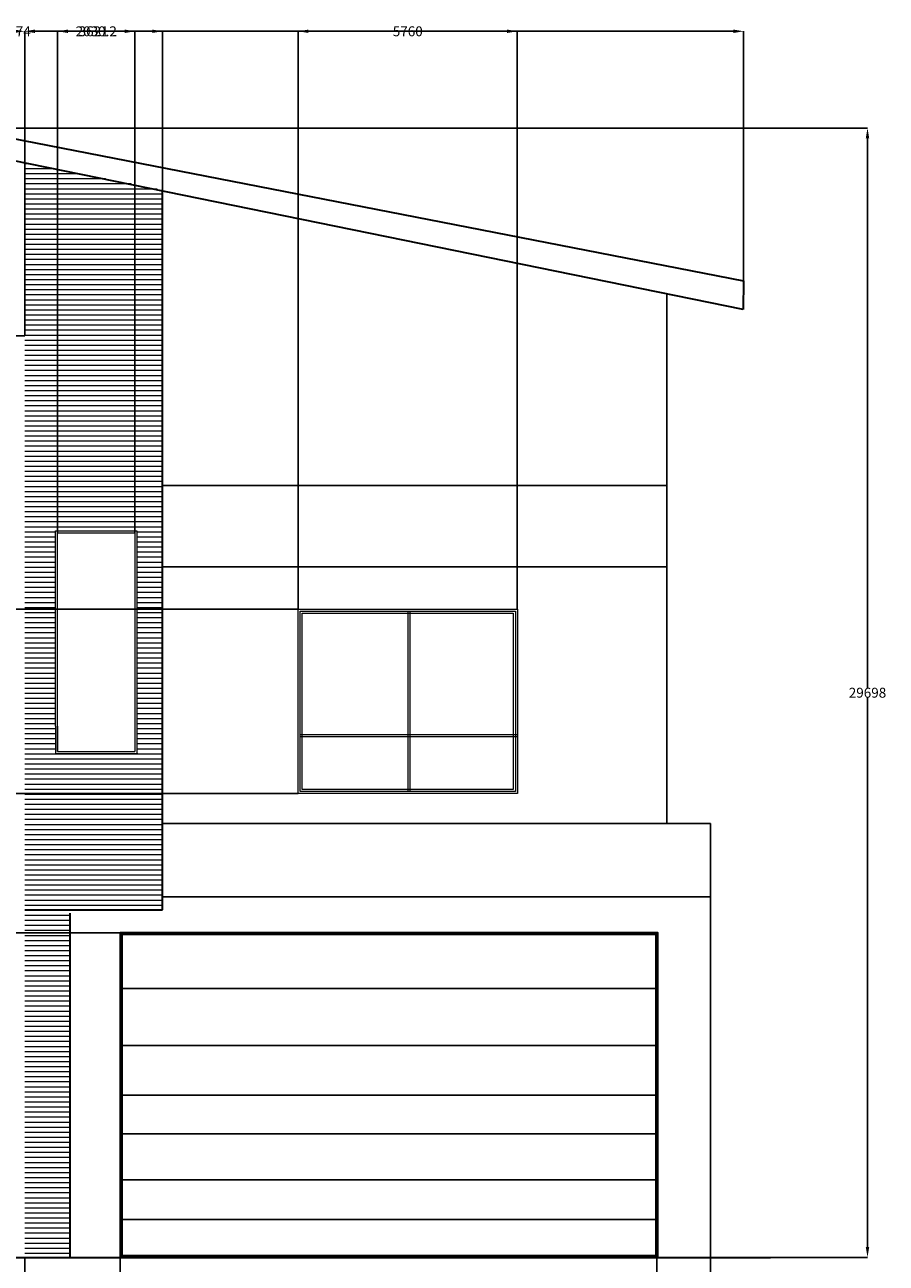
# Model space of a CAD drawing. Units: millimetres. Extents: x 23 to 3809233, y 4 to 290343.
# Tile 8 of 8: x 1921861 to 1944512, y 173128 to 205695. Entities that reach past the tile are written whole.
import ezdxf

# ---------------------------------------------------------------- set-up
doc = ezdxf.new("R2010")
doc.units = ezdxf.units.MM
doc.header["$MEASUREMENT"] = 0
for name, color, linetype, lineweight in [('A-ANNO-DIMS', 2, 'Continuous', 18), ('A-COLS', 7, 'Continuous', 35), ('A-DOOR', 3, 'Continuous', 25), ('A-ELEV', 7, 'Continuous', 25), ('A-ELEV-GRND', 7, 'Continuous', 30), ('A-GLAZ', 4, 'Continuous', 18), ('A-ROOF', 7, 'Continuous', 35), ('A-WALL-PATT', 252, 'Continuous', 13)]:
    doc.layers.add(name, color=color, linetype=linetype, lineweight=lineweight)
doc.styles.get("Standard").update_dxf_attribs({"font": 'arial.ttf'})
doc.dimstyles.get("Standard").update_dxf_attribs({"dimtxt": 260.18, "dimasz": 270.18, "dimexe": 0.18, "dimexo": 0.0625, "dimgap": 0.09, "dimtad": 0, "dimtih": 1, "dimtoh": 1, "dimdec": 0, "dimzin": 0, "dimdsep": 46, "dimtxsty": 'Standard', "dimcen": 0.09, "dimadec": 0, "dimazin": 0, "dimtfac": 1, "dimtdec": 0, "dimtofl": 0, "dimtmove": 0, "dimatfit": 3, "dimfxl": 1, "dimtolj": 1, "dimtzin": 0, "dimarcsym": 0})

# ---------------------------------------------------------------- blocks, each defined once
blk = doc.blocks.new('*D94')
at = {"layer": 'A-ANNO-DIMS', "color": 0, "lineweight": -2, "transparency": 16777216}
for p, q in [((1902289, 186535), (1902289, 205525)), ((1902560, 205524), (1921037, 205524)), ((1940493, 205524), (1922015, 205524)), ((1940763, 198959), (1940763, 205525))]:
    blk.add_line(p, q, dxfattribs=at)
at = {"layer": 'A-ANNO-DIMS', "color": 0, "transparency": 16777216}
for points in [[(1902560, 205569), (1902560, 205479), (1902289, 205524)], [(1940493, 205569), (1940493, 205479), (1940763, 205524)]]:
    blk.add_solid(points, dxfattribs=at)
at = {"layer": 'Defpoints', "color": 0, "transparency": 16777216}
for p in [(1940763, 205524), (1940763, 198959), (1902289, 186535)]:
    blk.add_point(p, dxfattribs=at)
at = {"layer": 'A-ANNO-DIMS', "color": 0, "transparency": 16777216, "insert": (1921526, 205524), "char_height": 260.2, "attachment_point": 5}
blk.add_mtext('\\A1;38474', dxfattribs=at)
blk = doc.blocks.new('*D95')
at = {"layer": 'A-ANNO-DIMS', "color": 0, "lineweight": -2, "transparency": 16777216}
for p, q in [((1920137, 202978), (1944019, 202978)), ((1944019, 202708), (1944019, 188263)), ((1944019, 173551), (1944019, 187997)), ((1939891, 173281), (1944019, 173281))]:
    blk.add_line(p, q, dxfattribs=at)
at = {"layer": 'A-ANNO-DIMS', "color": 0, "transparency": 16777216}
for points in [[(1943974, 202708), (1944064, 202708), (1944019, 202978)], [(1943974, 173551), (1944064, 173551), (1944019, 173281)]]:
    blk.add_solid(points, dxfattribs=at)
at = {"layer": 'Defpoints', "color": 0, "transparency": 16777216}
for p in [(1920137, 202978), (1944019, 202978), (1939891, 173281)]:
    blk.add_point(p, dxfattribs=at)
at = {"layer": 'A-ANNO-DIMS', "color": 0, "transparency": 16777216, "insert": (1944019, 188130), "char_height": 260.2, "attachment_point": 5}
blk.add_mtext('\\A1;29698', dxfattribs=at)
blk = doc.blocks.new('*D99')
at = {"layer": 'A-ANNO-DIMS', "color": 0, "lineweight": -2, "transparency": 16777216}
for p, q in [((1921861, 173281), (1921861, 166038)), ((1924370, 173282), (1924370, 166038)), ((1922131, 166038), (1922572, 166038)), ((1924100, 166038), (1923659, 166038))]:
    blk.add_line(p, q, dxfattribs=at)
at = {"layer": 'A-ANNO-DIMS', "color": 0, "transparency": 16777216}
for points in [[(1922131, 166083), (1922131, 165993), (1921861, 166038)], [(1924100, 166083), (1924100, 165993), (1924370, 166038)]]:
    blk.add_solid(points, dxfattribs=at)
at = {"layer": 'Defpoints', "color": 0, "transparency": 16777216}
for p in [(1921861, 173281), (1924370, 173282), (1924370, 166038)]:
    blk.add_point(p, dxfattribs=at)
at = {"layer": 'A-ANNO-DIMS', "color": 0, "transparency": 16777216, "insert": (1923116, 166038), "char_height": 260.2, "attachment_point": 5}
blk.add_mtext('\\A1;2509.5', dxfattribs=at)
blk = doc.blocks.new('*D100')
at = {"layer": 'A-ANNO-DIMS', "color": 0, "lineweight": -2, "transparency": 16777216}
for p, q in [((1924370, 173282), (1924370, 166038)), ((1938484, 173307), (1938484, 166038)), ((1924641, 166038), (1930950, 166038)), ((1938214, 166038), (1931904, 166038))]:
    blk.add_line(p, q, dxfattribs=at)
at = {"layer": 'A-ANNO-DIMS', "color": 0, "transparency": 16777216}
for points in [[(1924641, 166083), (1924641, 165993), (1924370, 166038)], [(1938214, 166083), (1938214, 165993), (1938484, 166038)]]:
    blk.add_solid(points, dxfattribs=at)
at = {"layer": 'Defpoints', "color": 0, "transparency": 16777216}
for p in [(1924370, 173282), (1938484, 173307), (1938484, 166038)]:
    blk.add_point(p, dxfattribs=at)
at = {"layer": 'A-ANNO-DIMS', "color": 0, "transparency": 16777216, "insert": (1931427, 166038), "char_height": 260.2, "attachment_point": 5}
blk.add_mtext('\\A1;14114', dxfattribs=at)
blk = doc.blocks.new('*D101')
at = {"layer": 'A-ANNO-DIMS', "color": 0, "lineweight": -2, "transparency": 16777216}
for p, q in [((1938484, 173307), (1938484, 166038)), ((1939891, 173281), (1939891, 166038)), ((1938214, 166038), (1937944, 166038)), ((1940162, 166038), (1940432, 166038))]:
    blk.add_line(p, q, dxfattribs=at)
at = {"layer": 'A-ANNO-DIMS', "color": 0, "transparency": 16777216}
for points in [[(1938214, 166083), (1938214, 165993), (1938484, 166038)], [(1940162, 166083), (1940162, 165993), (1939891, 166038)]]:
    blk.add_solid(points, dxfattribs=at)
at = {"layer": 'Defpoints', "color": 0, "transparency": 16777216}
for p in [(1938484, 173307), (1939891, 173281), (1939891, 166038)]:
    blk.add_point(p, dxfattribs=at)
at = {"layer": 'A-ANNO-DIMS', "color": 0, "transparency": 16777216, "insert": (1939188, 166038), "char_height": 260.2, "attachment_point": 5}
blk.add_mtext('\\A1;1407.4', dxfattribs=at)
blk = doc.blocks.new('*D104')
at = {"layer": 'A-ANNO-DIMS', "color": 0, "lineweight": -2, "transparency": 16777216}
for p, q in [((1924370.307623, 181820.425276), (1888189.886131, 181820.425276)), ((1888190.066131, 181550.245276), (1888190.066131, 177684.406757)), ((1888190.066131, 173552.529002), (1888190.066131, 177418.367521)), ((1924370.346212, 173282.349002), (1888189.886131, 173282.349002))]:
    blk.add_line(p, q, dxfattribs=at)
at = {"layer": 'A-ANNO-DIMS', "color": 0, "transparency": 16777216}
for points in [[(1888145.036131, 181550.245276), (1888235.096131, 181550.245276), (1888190.066131, 181820.425276)], [(1888145.036131, 173552.529002), (1888235.096131, 173552.529002), (1888190.066131, 173282.349002)]]:
    blk.add_solid(points, dxfattribs=at)
at = {"layer": 'Defpoints', "color": 0, "transparency": 16777216}
for p in [(1888190.066131, 181820.425276), (1924370.370123, 181820.425276), (1924370.408712, 173282.349002)]:
    blk.add_point(p, dxfattribs=at)
at = {"layer": 'A-ANNO-DIMS', "color": 0, "transparency": 16777216, "insert": (1888190.066131, 177551.387139), "char_height": 260.18, "attachment_point": 5}
blk.add_mtext('\\A1;8538', dxfattribs=at)
blk = doc.blocks.new('*D105')
at = {"layer": 'A-ANNO-DIMS', "color": 0, "lineweight": -2, "transparency": 16777216}
for p, q in [((1903366, 194022), (1903366, 205525)), ((1903636, 205524), (1912135, 205524)), ((1921591, 205524), (1913092, 205524)), ((1921861, 197518), (1921861, 205525))]:
    blk.add_line(p, q, dxfattribs=at)
at = {"layer": 'A-ANNO-DIMS', "color": 0, "transparency": 16777216}
for points in [[(1903636, 205569), (1903636, 205479), (1903366, 205524)], [(1921591, 205569), (1921591, 205479), (1921861, 205524)]]:
    blk.add_solid(points, dxfattribs=at)
at = {"layer": 'Defpoints', "color": 0, "transparency": 16777216}
for p in [(1921861, 205524), (1921861, 197518), (1903366, 194022)]:
    blk.add_point(p, dxfattribs=at)
at = {"layer": 'A-ANNO-DIMS', "color": 0, "transparency": 16777216, "insert": (1912613, 205524), "char_height": 260.2, "attachment_point": 5}
blk.add_mtext('\\A1;18495', dxfattribs=at)
blk = doc.blocks.new('*D106')
at = {"layer": 'A-ANNO-DIMS', "color": 0, "lineweight": -2, "transparency": 16777216}
for p, q in [((1921861, 197518), (1921861, 205525)), ((1922131, 205524), (1923308, 205524)), ((1925212, 205524), (1924035, 205524)), ((1925482, 201357), (1925482, 205525))]:
    blk.add_line(p, q, dxfattribs=at)
at = {"layer": 'A-ANNO-DIMS', "color": 0, "transparency": 16777216}
for points in [[(1922131, 205569), (1922131, 205479), (1921861, 205524)], [(1925212, 205569), (1925212, 205479), (1925482, 205524)]]:
    blk.add_solid(points, dxfattribs=at)
at = {"layer": 'Defpoints', "color": 0, "transparency": 16777216}
for p in [(1925482, 205524), (1925482, 201357), (1921861, 197518)]:
    blk.add_point(p, dxfattribs=at)
at = {"layer": 'A-ANNO-DIMS', "color": 0, "transparency": 16777216, "insert": (1923671, 205524), "char_height": 260.2, "attachment_point": 5}
blk.add_mtext('\\A1;3621', dxfattribs=at)
blk = doc.blocks.new('*D107')
at = {"layer": 'A-ANNO-DIMS', "color": 0, "lineweight": -2, "transparency": 16777216}
for p, q in [((1921861, 197518), (1888190, 197518)), ((1888190, 197248), (1888190, 195903)), ((1888190, 194292), (1888190, 195637)), ((1903366, 194022), (1888190, 194022))]:
    blk.add_line(p, q, dxfattribs=at)
at = {"layer": 'A-ANNO-DIMS', "color": 0, "transparency": 16777216}
for points in [[(1888145, 197248), (1888235, 197248), (1888190, 197518)], [(1888145, 194292), (1888235, 194292), (1888190, 194022)]]:
    blk.add_solid(points, dxfattribs=at)
at = {"layer": 'Defpoints', "color": 0, "transparency": 16777216}
for p in [(1888190, 197518), (1921861, 197518), (1903366, 194022)]:
    blk.add_point(p, dxfattribs=at)
at = {"layer": 'A-ANNO-DIMS', "color": 0, "transparency": 16777216, "insert": (1888190, 195770), "char_height": 260.2, "attachment_point": 5}
blk.add_mtext('\\A1;3496.4', dxfattribs=at)
blk = doc.blocks.new('*D113')
at = {"layer": 'A-ANNO-DIMS', "color": 0, "lineweight": -2, "transparency": 16777216}
for p, q in [((1922725, 192331), (1922725, 205525)), ((1922996, 205524), (1923199, 205524)), ((1924485, 205524), (1924282, 205524)), ((1924756, 192331), (1924756, 205525))]:
    blk.add_line(p, q, dxfattribs=at)
at = {"layer": 'A-ANNO-DIMS', "color": 0, "transparency": 16777216}
for points in [[(1922996, 205569), (1922996, 205479), (1922725, 205524)], [(1924485, 205569), (1924485, 205479), (1924756, 205524)]]:
    blk.add_solid(points, dxfattribs=at)
at = {"layer": 'Defpoints', "color": 0, "transparency": 16777216}
for p in [(1924756, 205524), (1922725, 192331), (1924756, 192331)]:
    blk.add_point(p, dxfattribs=at)
at = {"layer": 'A-ANNO-DIMS', "color": 0, "transparency": 16777216, "insert": (1923740, 205524), "char_height": 260.2, "attachment_point": 5}
blk.add_mtext('\\A1;2030.2', dxfattribs=at)
blk = doc.blocks.new('*D114')
at = {"layer": 'A-ANNO-DIMS', "color": 0, "lineweight": -2, "transparency": 16777216}
for p, q in [((1929050, 190325), (1929050, 205525)), ((1929321, 205524), (1931542, 205524)), ((1934541, 205524), (1932319, 205524)), ((1934811, 190327), (1934811, 205525))]:
    blk.add_line(p, q, dxfattribs=at)
at = {"layer": 'A-ANNO-DIMS', "color": 0, "transparency": 16777216}
for points in [[(1929321, 205569), (1929321, 205479), (1929050, 205524)], [(1934541, 205569), (1934541, 205479), (1934811, 205524)]]:
    blk.add_solid(points, dxfattribs=at)
at = {"layer": 'Defpoints', "color": 0, "transparency": 16777216}
for p in [(1934811, 205524), (1929050, 190325), (1934811, 190327)]:
    blk.add_point(p, dxfattribs=at)
at = {"layer": 'A-ANNO-DIMS', "color": 0, "transparency": 16777216, "insert": (1931931, 205524), "char_height": 260.2, "attachment_point": 5}
blk.add_mtext('\\A1;5760', dxfattribs=at)
blk = doc.blocks.new('*D115')
at = {"layer": 'A-ANNO-DIMS', "color": 0, "lineweight": -2, "transparency": 16777216}
for p, q in [((1929050.318541, 190325.231012), (1888189.886131, 190325.231012)), ((1888190.066131, 190055.051012), (1888190.066131, 188036.972999)), ((1888190.066131, 185752.85575), (1888190.066131, 187770.933763)), ((1929050.318541, 185482.67575), (1888189.886131, 185482.67575))]:
    blk.add_line(p, q, dxfattribs=at)
at = {"layer": 'A-ANNO-DIMS', "color": 0, "transparency": 16777216}
for points in [[(1888145.036131, 190055.051012), (1888235.096131, 190055.051012), (1888190.066131, 190325.231012)], [(1888145.036131, 185752.85575), (1888235.096131, 185752.85575), (1888190.066131, 185482.67575)]]:
    blk.add_solid(points, dxfattribs=at)
at = {"layer": 'Defpoints', "color": 0, "transparency": 16777216}
for p in [(1888190.066131, 190325.231012), (1929050.381041, 190325.231012), (1929050.381041, 185482.67575)]:
    blk.add_point(p, dxfattribs=at)
at = {"layer": 'A-ANNO-DIMS', "color": 0, "transparency": 16777216, "insert": (1888190.066131, 187903.953381), "char_height": 260.18, "attachment_point": 5}
blk.add_mtext('\\A1;4843', dxfattribs=at)

msp = doc.modelspace()

# ---------------------------------------------------------------- hatches: boundary and pattern name
at = {"layer": 'A-WALL-PATT'}
h = msp.add_hatch(dxfattribs=at)
h.set_pattern_fill('ANSI31', color=256, scale=1061.3134, angle=-45, style=0)
h.paths.add_polyline_path([(1921860.931, 182422.235), (1925481.709, 182422.235), (1925481.709, 201356.818), (1921860.931, 202063.759)])
h.paths.add_polyline_path([(1922672.309, 192384.187), (1924806.696, 192384.187), (1924806.696, 186534.824), (1922672.309, 186534.824)], flags=0)
h = msp.add_hatch(dxfattribs=at)
h.set_pattern_fill('ANSI31', color=256, scale=1061.3134, angle=-45, style=0)
h.paths.add_polyline_path([(1921860.931, 173280.749), (1923056.615, 173280.749), (1923056.615, 182422.235), (1921860.931, 182422.235)])

# ---------------------------------------------------------------- linework, layer by layer
at = {"layer": 'A-COLS'}
for p, q in [((1925481.709, 195073.74), (1925481.709, 201356.818)), ((1925481.709, 182422.235), (1925481.709, 195073.74)), ((1921860.931, 182422.235), (1925481.709, 182422.235)), ((1923056.615, 173280.749), (1923056.615, 182330.475))]:
    msp.add_line(p, q, dxfattribs=at)
at = {"layer": 'A-DOOR'}
for p, q in [((1924423.436, 180352.795), (1938510.519, 180352.795)), ((1924370.37, 178855.255), (1938510.519, 178855.255)), ((1924423.436, 177551.582), (1938510.519, 177551.582)), ((1924396.903, 176534.585), (1938457.453, 176534.585)), ((1924396.903, 175317.891), (1938510.519, 175317.891)), ((1924423.436, 174280.085), (1938510.519, 174280.085))]:
    msp.add_line(p, q, dxfattribs=at)
msp.add_lwpolyline([(1938510.519, 173282.739, -0.414213562), (1938508.529, 173280.749), (1924372.36, 173280.749, -0.414213562), (1924370.37, 173282.739), (1924370.37, 181820.425, -0.414213562), (1924372.36, 181822.415), (1938508.529, 181822.415, -0.414213562), (1938510.519, 181820.425)], format="xyb", close=True, dxfattribs=at)
for points in [[(1938483.986, 173307.282), (1924396.903, 173307.282), (1924396.903, 181795.882), (1938483.986, 181795.882)], [(1938457.453, 173333.815), (1924423.436, 173333.815), (1924423.436, 181769.35), (1938457.453, 181769.35)]]:
    msp.add_lwpolyline(points, close=True, dxfattribs=at)
at = {"layer": 'A-ELEV'}
for p, q in [((1938740.781, 193575.546), (1938740.781, 198617.113)), ((1938740.781, 193575.546), (1925481.709, 193575.546)), ((1938740.781, 184691.073), (1938740.781, 193575.546)), ((1928568.226, 184677.526), (1928570.216, 184677.526)), ((1939891.392, 182760.245), (1925481.709, 182760.245)), ((1939891.392, 173280.749), (1939891.392, 182760.245))]:
    msp.add_line(p, q, dxfattribs=at)
msp.add_lwpolyline([(1925481.709, 191443.399), (1925481.709, 191443.399), (1938740.781, 191443.399), (1938740.781, 191443.399), (1938740.781, 191443.399), (1938740.781, 191443.399), (1925481.709, 191443.399), (1925481.709, 191443.399)], close=True, dxfattribs=at)
for points in [[(1925481.709, 184691.073), (1939889.402, 184691.073, -0.414213562), (1939891.392, 184689.083), (1939891.392, 182762.235, -0.414213562), (1939889.402, 182760.245)], [(1928572.205, 184691.073, -0.414213562), (1928570.216, 184693.063)]]:
    msp.add_lwpolyline(points, format="xyb", dxfattribs=at)
at = {"layer": 'A-ELEV-GRND'}
msp.add_line((1914495.5, 173280.749), (1941473.027, 173280.749), dxfattribs=at)
at = {"layer": 'A-GLAZ'}
for p, q in [((1924753.63, 192331.121), (1924753.63, 186587.89)), ((1931931.582, 190274.155), (1931931.582, 185533.751)), ((1931984.647, 190274.155), (1931984.647, 185533.751)), ((1922672.309, 187248.079), (1922672.309, 186534.824)), ((1922725.374, 187248.079), (1922725.374, 186587.89)), ((1924806.696, 187246.089), (1924806.696, 186534.824)), ((1929103.447, 187035.053), (1934812.782, 187035.053)), ((1929103.447, 186981.987), (1934812.782, 186981.987)), ((1922672.309, 186534.824), (1924832.632, 186534.824)), ((1922725.374, 186587.89), (1924753.63, 186587.89))]:
    msp.add_line(p, q, dxfattribs=at)
msp.add_lwpolyline([(1922674.298, 187246.089, -0.414213562), (1922672.309, 187248.079), (1922672.309, 192382.197, -0.414213562), (1922674.298, 192384.187), (1924806.696, 192384.187, -0.414213562), (1924808.686, 192382.197), (1924808.686, 187248.079, -0.414213562), (1924806.696, 187246.089)], format="xyb", dxfattribs=at)
msp.add_lwpolyline([(1922725.374, 186587.89), (1922725.374, 192331.121), (1924755.62, 192331.121), (1924755.62, 187299.154)], dxfattribs=at)
msp.add_lwpolyline([(1929050.381, 190325.231, -0.414213562), (1929052.371, 190327.221), (1934810.792, 190327.221, -0.414213562), (1934812.782, 190325.231), (1934812.782, 185482.676, -0.414213562), (1934810.792, 185480.686), (1929052.371, 185480.686, -0.414213562), (1929050.381, 185482.676)], format="xyb", close=True, dxfattribs=at)
for points in [[(1929103.447, 190274.155), (1934759.717, 190274.155), (1934759.717, 185533.751), (1929103.447, 185533.751)], [(1929156.512, 190221.09), (1934706.651, 190221.09), (1934706.651, 185586.817), (1929156.512, 185586.817)]]:
    msp.add_lwpolyline(points, close=True, dxfattribs=at)
at = {"layer": 'A-ROOF'}
for p, q in [((1920136.86, 202978.465), (1940762.989, 198959.058)), ((1940749.627, 198207.142), (1920136.86, 202413.849)), ((1938740.781, 199353.125), (1938740.781, 199366.95)), ((1940762.989, 198959.058), (1940749.627, 198207.142))]:
    msp.add_line(p, q, dxfattribs=at)

# ---------------------------------------------------------------- dimensions: what is measured, and where the dimension line sits
at = {"layer": 'A-ANNO-DIMS'}
for base, p1, p2, override, picture, middle in [((1940762.989, 205524.465), (1902289.394, 186534.824), (1940762.989, 198959.058), {"dimdec": 0, "dimlfac": 1, "dimrnd": 0, "dimzin": 0, "dimdsep": 46, "dimlunit": 2}, '*D94', (1921526.192, 205524.465)), ((1921860.931, 205524.465), (1903365.563, 194021.715), (1921860.931, 197518.123), {"dimdec": 0, "dimlfac": 1, "dimrnd": 0, "dimzin": 0, "dimdsep": 46, "dimlunit": 2}, '*D105', (1912613.247, 205524.465)), ((1925481.709, 205524.465), (1921860.931, 197518.123), (1925481.709, 201356.818), {"dimdec": 0, "dimlfac": 1, "dimrnd": 0, "dimzin": 0, "dimdsep": 46, "dimlunit": 2}, '*D106', (1923671.32, 205524.465)), ((1924755.62, 205524.465), (1922725.374, 192331.121), (1924755.62, 192331.121), {"dimdec": 1, "dimlfac": 1, "dimrnd": 0, "dimzin": 0, "dimdsep": 46, "dimlunit": 2}, '*D113', (1923740.497, 205524.465)), ((1934810.792, 205524.465), (1929050.381, 190325.231), (1934810.792, 190327.221), {"dimdec": 0, "dimlfac": 1, "dimrnd": 0, "dimzin": 0, "dimdsep": 46, "dimlunit": 2}, '*D114', (1931930.587, 205524.465)), ((1924370.409, 166037.69), (1921860.931, 173280.749), (1924370.409, 173282.349), {"dimdec": 1, "dimlfac": 1, "dimrnd": 0, "dimzin": 0, "dimdsep": 46, "dimlunit": 2}, '*D99', (1923115.67, 166037.69)), ((1938483.986, 166037.69), (1924370.409, 173282.349), (1938483.986, 173307.282), {"dimdec": 0, "dimlfac": 1, "dimrnd": 0, "dimzin": 0, "dimdsep": 46, "dimlunit": 2}, '*D100', (1931427.197, 166037.69)), ((1939891.392, 166037.69), (1938483.986, 173307.282), (1939891.392, 173280.749), {"dimdec": 1, "dimlfac": 1, "dimrnd": 0, "dimzin": 0, "dimdsep": 46, "dimlunit": 2}, '*D101', (1939187.689, 166037.69))]:
    dim = msp.add_linear_dim(base=base, p1=p1, p2=p2, dimstyle='Standard', override=override, dxfattribs=at)
    dim.commit()
    dim.dimension.update_dxf_attribs({"geometry": picture, "text_midpoint": middle})
for base, p1, p2, override, picture, middle in [((1944019.027, 202978.465), (1939891.392, 173280.749), (1920136.86, 202978.465), {"dimdec": 0, "dimlfac": 1, "dimrnd": 0, "dimzin": 0, "dimdsep": 46, "dimlunit": 2}, '*D95', (1944019.027, 188129.607)), ((1888190.066, 197518.123), (1903365.563, 194021.715), (1921860.931, 197518.123), {"dimdec": 1, "dimlfac": 1, "dimrnd": 0, "dimzin": 0, "dimdsep": 46, "dimlunit": 2}, '*D107', (1888190.066, 195769.919)), ((1888190.066, 190325.231), (1929050.381, 185482.676), (1929050.381, 190325.231), {"dimdec": 0, "dimlfac": 1, "dimrnd": 0, "dimzin": 0, "dimdsep": 46, "dimlunit": 2}, '*D115', (1888190.066, 187903.953)), ((1888190.066, 181820.425), (1924370.409, 173282.349), (1924370.37, 181820.425), {"dimdec": 0, "dimlfac": 1, "dimrnd": 0, "dimzin": 0, "dimdsep": 46, "dimlunit": 2}, '*D104', (1888190.066, 177551.387))]:
    dim = msp.add_linear_dim(base=base, p1=p1, p2=p2, angle=90, dimstyle='Standard', override=override, dxfattribs=at)
    dim.commit()
    dim.dimension.update_dxf_attribs({"geometry": picture, "text_midpoint": middle})

doc.saveas('drawing.dxf')
